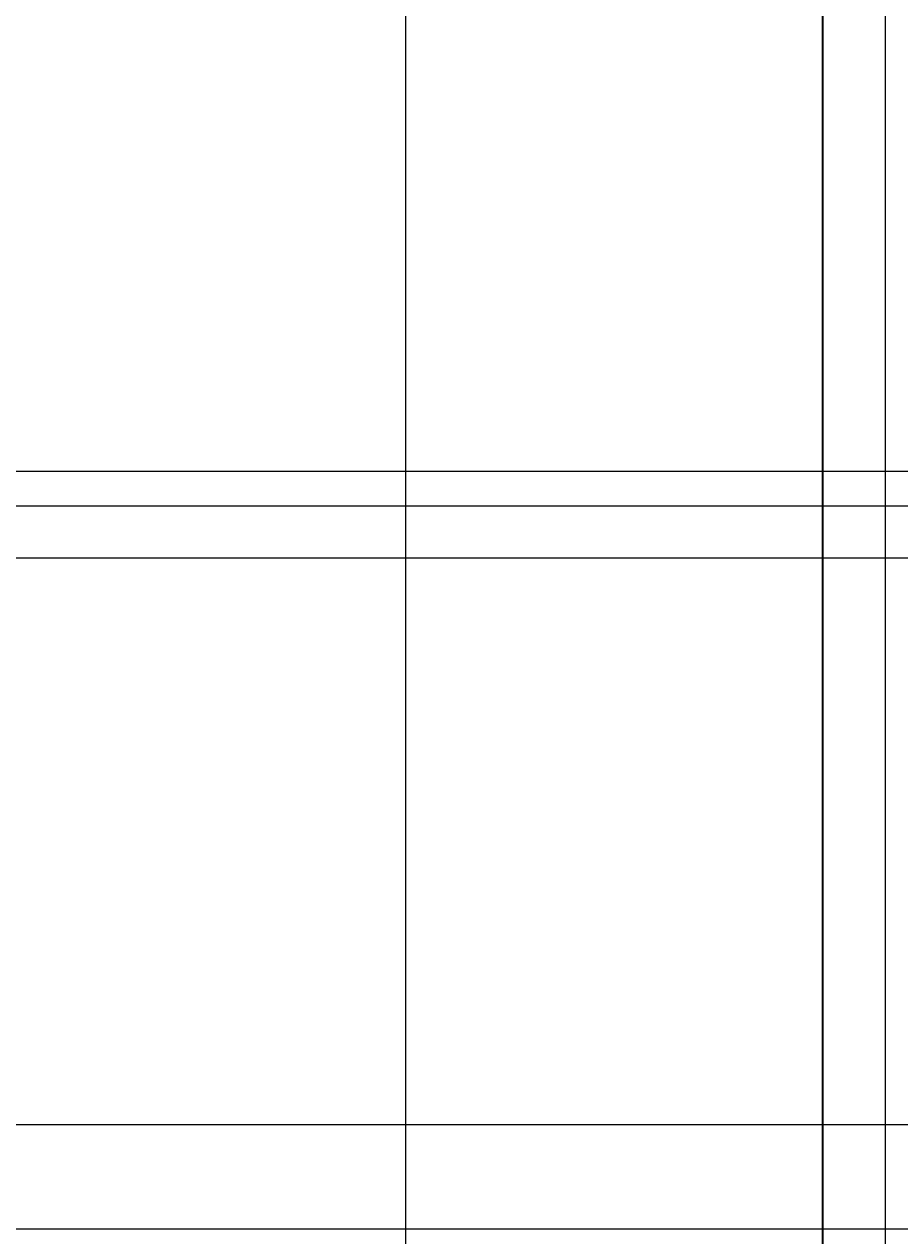
# Model space of a CAD drawing. Units: inches. Extents: x -6 to 289, y -8 to 323.
# Tile 73 of 107: x 248 to 273, y 159 to 194. Entities that reach past the tile are written whole.
import ezdxf

# ---------------------------------------------------------------- set-up
doc = ezdxf.new("R2010")
doc.units = ezdxf.units.IN
doc.header["$MEASUREMENT"] = 0
doc.layers.add('A-ANNO-DIMS', color=2, linetype='Continuous', lineweight=18)
doc.layers.add('A-ELEV', color=7, linetype='Continuous', lineweight=35)
doc.styles.get("Standard").update_dxf_attribs({"font": 'arial.ttf'})
doc.dimstyles.get("Standard").update_dxf_attribs({"dimtxt": 0.18, "dimasz": 0.18, "dimexe": 0.18, "dimexo": 0.0625, "dimgap": 0.09, "dimtad": 0, "dimtih": 1, "dimtoh": 1, "dimdec": 4, "dimzin": 0, "dimdsep": 46, "dimtxsty": 'Standard', "dimcen": 0.09, "dimadec": 0, "dimazin": 0, "dimtfac": 1, "dimtdec": 4, "dimtofl": 0, "dimtmove": 0, "dimatfit": 3, "dimfxl": 1, "dimtolj": 1, "dimtzin": 0, "dimarcsym": 0})

# ---------------------------------------------------------------- blocks, each defined once
blk = doc.blocks.new('*D15')
at = {"layer": 'A-ANNO-DIMS', "color": 0, "lineweight": -2, "transparency": 16777216}
for p, q in [((247.164, 162.411), (247.164, 322.969)), ((271.164, 7.351), (271.164, 322.969)), ((247.344, 322.789), (258.944, 322.789)), ((270.984, 322.789), (259.384, 322.789))]:
    blk.add_line(p, q, dxfattribs=at)
at = {"layer": 'A-ANNO-DIMS', "color": 0, "transparency": 16777216}
for points in [[(247.344, 322.819), (247.344, 322.759), (247.164, 322.789)], [(270.984, 322.819), (270.984, 322.759), (271.164, 322.789)]]:
    blk.add_solid(points, dxfattribs=at)
at = {"layer": 'Defpoints', "color": 0, "transparency": 16777216}
for p in [(271.164, 322.789), (247.164, 162.348), (271.164, 7.289)]:
    blk.add_point(p, dxfattribs=at)
at = {"layer": 'A-ANNO-DIMS', "color": 0, "transparency": 16777216, "insert": (259.164, 322.789), "char_height": 0.18, "attachment_point": 5}
blk.add_mtext('\\A1;24', dxfattribs=at)
blk = doc.blocks.new('*D24')
at = {"layer": 'A-ANNO-DIMS', "color": 0, "lineweight": -2, "transparency": 16777216}
for p, q in [((126.946, 178.654), (288.653, 178.654)), ((288.473, 178.474), (288.473, 159.153)), ((288.473, 139.469), (288.473, 158.789)), ((259.226, 139.289), (288.653, 139.289))]:
    blk.add_line(p, q, dxfattribs=at)
at = {"layer": 'A-ANNO-DIMS', "color": 0, "transparency": 16777216}
for points in [[(288.443, 178.474), (288.503, 178.474), (288.473, 178.654)], [(288.443, 139.469), (288.503, 139.469), (288.473, 139.289)]]:
    blk.add_solid(points, dxfattribs=at)
at = {"layer": 'Defpoints', "color": 0, "transparency": 16777216}
for p in [(126.883, 178.654), (288.473, 178.654), (259.164, 139.289)]:
    blk.add_point(p, dxfattribs=at)
at = {"layer": 'A-ANNO-DIMS', "color": 0, "transparency": 16777216, "insert": (288.473, 158.971), "char_height": 0.18, "attachment_point": 5}
blk.add_mtext('\\A1;39.365', dxfattribs=at)
blk = doc.blocks.new('*D25')
at = {"layer": 'A-ANNO-DIMS', "color": 0, "lineweight": -2, "transparency": 16777216}
for p, q in [((126.946, 226.654), (288.653, 226.654)), ((288.473, 226.474), (288.473, 202.836)), ((288.473, 178.834), (288.473, 202.472)), ((126.946, 178.654), (288.653, 178.654))]:
    blk.add_line(p, q, dxfattribs=at)
at = {"layer": 'A-ANNO-DIMS', "color": 0, "transparency": 16777216}
for points in [[(288.443, 226.474), (288.503, 226.474), (288.473, 226.654)], [(288.443, 178.834), (288.503, 178.834), (288.473, 178.654)]]:
    blk.add_solid(points, dxfattribs=at)
at = {"layer": 'Defpoints', "color": 0, "transparency": 16777216}
for p in [(126.883, 226.654), (288.473, 226.654), (126.883, 178.654)]:
    blk.add_point(p, dxfattribs=at)
at = {"layer": 'A-ANNO-DIMS', "color": 0, "transparency": 16777216, "insert": (288.473, 202.654), "char_height": 0.18, "attachment_point": 5}
blk.add_mtext('\\A1;48', dxfattribs=at)
blk = doc.blocks.new('*D35')
at = {"layer": 'A-ANNO-DIMS', "color": 0, "lineweight": -2, "transparency": 16777216}
for p, q in [((167.446, 180.154), (288.653, 180.154)), ((288.473, 179.974), (288.473, 179.586)), ((288.473, 178.834), (288.473, 179.222)), ((168.946, 178.654), (288.653, 178.654))]:
    blk.add_line(p, q, dxfattribs=at)
at = {"layer": 'A-ANNO-DIMS', "color": 0, "transparency": 16777216}
for points in [[(288.443, 179.974), (288.503, 179.974), (288.473, 180.154)], [(288.443, 178.834), (288.503, 178.834), (288.473, 178.654)]]:
    blk.add_solid(points, dxfattribs=at)
at = {"layer": 'Defpoints', "color": 0, "transparency": 16777216}
for p in [(167.383, 180.154), (288.473, 180.154), (168.883, 178.654)]:
    blk.add_point(p, dxfattribs=at)
at = {"layer": 'A-ANNO-DIMS', "color": 0, "transparency": 16777216, "insert": (288.473, 179.404), "char_height": 0.18, "attachment_point": 5}
blk.add_mtext('\\A1;1.5', dxfattribs=at)
blk = doc.blocks.new('*D36')
at = {"layer": 'A-ANNO-DIMS', "color": 0, "lineweight": -2, "transparency": 16777216}
for p, q in [((166.446, 181.154), (288.653, 181.154)), ((288.473, 180.974), (288.473, 180.834)), ((288.473, 180.334), (288.473, 180.474)), ((167.446, 180.154), (288.653, 180.154))]:
    blk.add_line(p, q, dxfattribs=at)
at = {"layer": 'A-ANNO-DIMS', "color": 0, "transparency": 16777216}
for points in [[(288.443, 180.974), (288.503, 180.974), (288.473, 181.154)], [(288.443, 180.334), (288.503, 180.334), (288.473, 180.154)]]:
    blk.add_solid(points, dxfattribs=at)
at = {"layer": 'Defpoints', "color": 0, "transparency": 16777216}
for p in [(166.383, 181.154), (288.473, 181.154), (167.383, 180.154)]:
    blk.add_point(p, dxfattribs=at)
at = {"layer": 'A-ANNO-DIMS', "color": 0, "transparency": 16777216, "insert": (288.473, 180.654), "char_height": 0.18, "attachment_point": 5}
blk.add_mtext('\\A1;1', dxfattribs=at)
blk = doc.blocks.new('*D37')
at = {"layer": 'A-ANNO-DIMS', "color": 0, "lineweight": -2, "transparency": 16777216}
for p, q in [((166.446, 224.154), (288.653, 224.154)), ((288.473, 223.974), (288.473, 202.836)), ((288.473, 181.334), (288.473, 202.472)), ((166.446, 181.154), (288.653, 181.154))]:
    blk.add_line(p, q, dxfattribs=at)
at = {"layer": 'A-ANNO-DIMS', "color": 0, "transparency": 16777216}
for points in [[(288.443, 223.974), (288.503, 223.974), (288.473, 224.154)], [(288.443, 181.334), (288.503, 181.334), (288.473, 181.154)]]:
    blk.add_solid(points, dxfattribs=at)
at = {"layer": 'Defpoints', "color": 0, "transparency": 16777216}
for p in [(166.383, 224.154), (288.473, 224.154), (166.383, 181.154)]:
    blk.add_point(p, dxfattribs=at)
at = {"layer": 'A-ANNO-DIMS', "color": 0, "transparency": 16777216, "insert": (288.473, 202.654), "char_height": 0.18, "attachment_point": 5}
blk.add_mtext('\\A1;43', dxfattribs=at)
blk = doc.blocks.new('*D47')
at = {"layer": 'A-ANNO-DIMS', "color": 0, "lineweight": -2, "transparency": 16777216}
for p, q in [((233.854, 224.389), (288.653, 224.389)), ((288.473, 224.209), (288.473, 193.55)), ((288.473, 162.528), (288.473, 193.187)), ((236.354, 162.348), (288.653, 162.348))]:
    blk.add_line(p, q, dxfattribs=at)
at = {"layer": 'A-ANNO-DIMS', "color": 0, "transparency": 16777216}
for points in [[(288.443, 224.209), (288.503, 224.209), (288.473, 224.389)], [(288.443, 162.528), (288.503, 162.528), (288.473, 162.348)]]:
    blk.add_solid(points, dxfattribs=at)
at = {"layer": 'Defpoints', "color": 0, "transparency": 16777216}
for p in [(233.792, 224.389), (288.473, 224.389), (236.292, 162.348)]:
    blk.add_point(p, dxfattribs=at)
at = {"layer": 'A-ANNO-DIMS', "color": 0, "transparency": 16777216, "insert": (288.473, 193.369), "char_height": 0.18, "attachment_point": 5}
blk.add_mtext('\\A1;62.04', dxfattribs=at)
blk = doc.blocks.new('*D82')
at = {"layer": 'A-ANNO-DIMS', "color": 0, "lineweight": -2, "transparency": 16777216}
for p, q in [((245.215, 66.286), (245.215, 322.969)), ((272.973, 66.286), (272.973, 322.969)), ((245.395, 322.789), (258.699, 322.789)), ((272.793, 322.789), (259.489, 322.789))]:
    blk.add_line(p, q, dxfattribs=at)
at = {"layer": 'A-ANNO-DIMS', "color": 0, "transparency": 16777216}
for points in [[(245.395, 322.819), (245.395, 322.759), (245.215, 322.789)], [(272.793, 322.819), (272.793, 322.759), (272.973, 322.789)]]:
    blk.add_solid(points, dxfattribs=at)
at = {"layer": 'Defpoints', "color": 0, "transparency": 16777216}
for p in [(272.973, 322.789), (245.215, 66.224), (272.973, 66.224)]:
    blk.add_point(p, dxfattribs=at)
at = {"layer": 'A-ANNO-DIMS', "color": 0, "transparency": 16777216, "insert": (259.094, 322.789), "char_height": 0.18, "attachment_point": 5}
blk.add_mtext('\\A1;27.76', dxfattribs=at)
blk = doc.blocks.new('*D100')
at = {"layer": 'A-ANNO-DIMS', "color": 0, "lineweight": -2, "transparency": 16777216}
for p, q in [((247.164, 162.411), (247.164, 322.969)), ((259.164, 139.351), (259.164, 322.969)), ((247.344, 322.789), (252.954, 322.789)), ((258.984, 322.789), (253.373, 322.789))]:
    blk.add_line(p, q, dxfattribs=at)
at = {"layer": 'A-ANNO-DIMS', "color": 0, "transparency": 16777216}
for points in [[(247.344, 322.819), (247.344, 322.759), (247.164, 322.789)], [(258.984, 322.819), (258.984, 322.759), (259.164, 322.789)]]:
    blk.add_solid(points, dxfattribs=at)
at = {"layer": 'Defpoints', "color": 0, "transparency": 16777216}
for p in [(259.164, 322.789), (247.164, 162.348), (259.164, 139.289)]:
    blk.add_point(p, dxfattribs=at)
at = {"layer": 'A-ANNO-DIMS', "color": 0, "transparency": 16777216, "insert": (253.164, 322.789), "char_height": 0.18, "attachment_point": 5}
blk.add_mtext('\\A1;12', dxfattribs=at)
blk = doc.blocks.new('*D103')
at = {"layer": 'A-ANNO-DIMS', "color": 0, "lineweight": -2, "transparency": 16777216}
for p, q in [((244.226, 159.348), (288.653, 159.348)), ((288.473, 159.168), (288.473, 151)), ((288.473, 142.469), (288.473, 150.637)), ((244.226, 142.289), (288.653, 142.289))]:
    blk.add_line(p, q, dxfattribs=at)
at = {"layer": 'A-ANNO-DIMS', "color": 0, "transparency": 16777216}
for points in [[(288.443, 159.168), (288.503, 159.168), (288.473, 159.348)], [(288.443, 142.469), (288.503, 142.469), (288.473, 142.289)]]:
    blk.add_solid(points, dxfattribs=at)
at = {"layer": 'Defpoints', "color": 0, "transparency": 16777216}
for p in [(244.164, 159.348), (288.473, 159.348), (244.164, 142.289)]:
    blk.add_point(p, dxfattribs=at)
at = {"layer": 'A-ANNO-DIMS', "color": 0, "transparency": 16777216, "insert": (288.473, 150.819), "char_height": 0.18, "attachment_point": 5}
blk.add_mtext('\\A1;17.06', dxfattribs=at)
blk = doc.blocks.new('*D104')
at = {"layer": 'A-ANNO-DIMS', "color": 0, "lineweight": -2, "transparency": 16777216}
for p, q in [((247.226, 162.348), (288.653, 162.348)), ((288.473, 162.168), (288.473, 161.03)), ((288.473, 159.528), (288.473, 160.666)), ((244.226, 159.348), (288.653, 159.348))]:
    blk.add_line(p, q, dxfattribs=at)
at = {"layer": 'A-ANNO-DIMS', "color": 0, "transparency": 16777216}
for points in [[(288.443, 162.168), (288.503, 162.168), (288.473, 162.348)], [(288.443, 159.528), (288.503, 159.528), (288.473, 159.348)]]:
    blk.add_solid(points, dxfattribs=at)
at = {"layer": 'Defpoints', "color": 0, "transparency": 16777216}
for p in [(247.164, 162.348), (288.473, 162.348), (244.164, 159.348)]:
    blk.add_point(p, dxfattribs=at)
at = {"layer": 'A-ANNO-DIMS', "color": 0, "transparency": 16777216, "insert": (288.473, 160.848), "char_height": 0.18, "attachment_point": 5}
blk.add_mtext('\\A1;3', dxfattribs=at)

msp = doc.modelspace()

# ---------------------------------------------------------------- linework, layer by layer
at = {"layer": 'A-ELEV'}
msp.add_line((271.1638, 68.4323), (271.1638, 259.2888), dxfattribs=at)

# ---------------------------------------------------------------- dimensions: what is measured, and where the dimension line sits
at = {"layer": 'A-ANNO-DIMS'}
for base, p1, p2, override, picture, middle in [((272.9733, 322.7888), (245.2146, 66.2238), (272.9733, 66.2238), {"dimdec": 2, "dimlfac": 1, "dimrnd": 0, "dimzin": 0, "dimdsep": 46, "dimlunit": 2}, '*D82', (259.0939, 322.7888)), ((271.1638, 322.7888), (247.1638, 162.3484), (271.1638, 7.2888), {"dimdec": 0, "dimlfac": 1, "dimrnd": 0, "dimzin": 0, "dimdsep": 46, "dimlunit": 2}, '*D15', (259.1638, 322.7888)), ((259.1638, 322.7888), (247.1638, 162.3484), (259.1638, 139.2888), {"dimdec": 0, "dimlfac": 1, "dimrnd": 0, "dimzin": 0, "dimdsep": 46, "dimlunit": 2}, '*D100', (253.1638, 322.7888))]:
    dim = msp.add_linear_dim(base=base, p1=p1, p2=p2, dimstyle='Standard', override=override, dxfattribs=at)
    dim.commit()
    dim.dimension.update_dxf_attribs({"geometry": picture, "text_midpoint": middle})
for base, p1, p2, override, picture, middle in [((288.4733, 226.654), (126.8835, 178.654), (126.8835, 226.654), {"dimdec": 0, "dimlfac": 1, "dimrnd": 0, "dimzin": 0, "dimdsep": 46, "dimlunit": 2}, '*D25', (288.4733, 202.654)), ((288.4733, 224.3887), (236.2918, 162.3484), (233.7918, 224.3887), {"dimdec": 2, "dimlfac": 1, "dimrnd": 0, "dimzin": 0, "dimdsep": 46, "dimlunit": 2}, '*D47', (288.4733, 193.3685)), ((288.4733, 224.154), (166.3835, 181.154), (166.3835, 224.154), {"dimdec": 0, "dimlfac": 1, "dimrnd": 0, "dimzin": 0, "dimdsep": 46, "dimlunit": 2}, '*D37', (288.4733, 202.654)), ((288.4733, 181.154), (167.3835, 180.154), (166.3835, 181.154), {"dimdec": 0, "dimlfac": 1, "dimrnd": 0, "dimzin": 0, "dimdsep": 46, "dimlunit": 2}, '*D36', (288.4733, 180.654)), ((288.4733, 180.154), (168.8835, 178.654), (167.3835, 180.154), {"dimdec": 1, "dimlfac": 1, "dimrnd": 0, "dimzin": 0, "dimdsep": 46, "dimlunit": 2}, '*D35', (288.4733, 179.404)), ((288.4733, 178.654), (259.1638, 139.2888), (126.8835, 178.654), {"dimdec": 3, "dimlfac": 1, "dimrnd": 0, "dimzin": 0, "dimdsep": 46, "dimlunit": 2}, '*D24', (288.4733, 158.9714)), ((288.4733, 162.3484), (244.1638, 159.3484), (247.1638, 162.3484), {"dimdec": 0, "dimlfac": 1, "dimrnd": 0, "dimzin": 0, "dimdsep": 46, "dimlunit": 2}, '*D104', (288.4733, 160.8484)), ((288.4733, 159.3484), (244.1638, 142.2888), (244.1638, 159.3484), {"dimdec": 2, "dimlfac": 1, "dimrnd": 0, "dimzin": 0, "dimdsep": 46, "dimlunit": 2}, '*D103', (288.4733, 150.8186))]:
    dim = msp.add_linear_dim(base=base, p1=p1, p2=p2, angle=90, dimstyle='Standard', override=override, dxfattribs=at)
    dim.commit()
    dim.dimension.update_dxf_attribs({"geometry": picture, "text_midpoint": middle})

doc.saveas('drawing.dxf')
